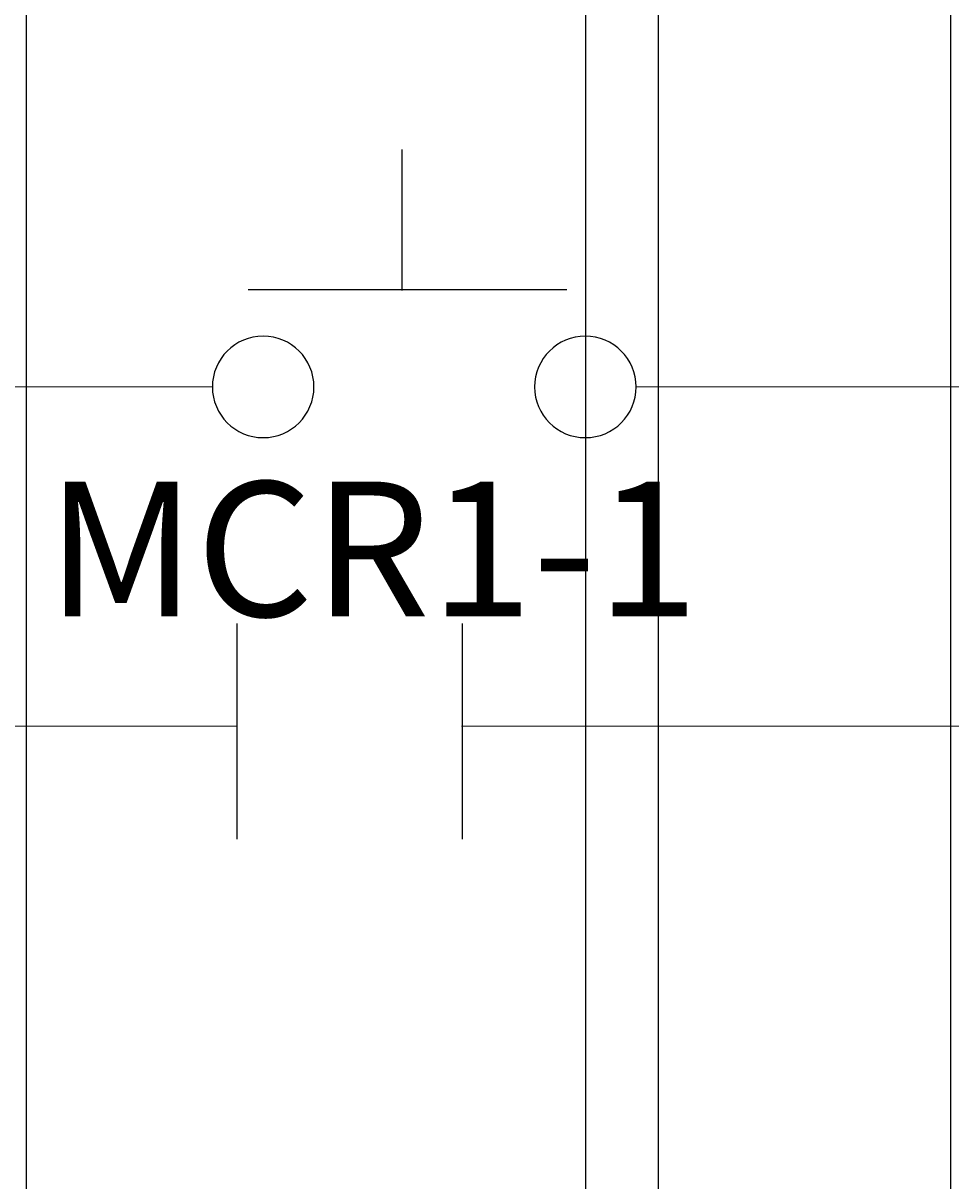
# Model space of a CAD drawing. Units: inches. Extents: x 738 to 1068, y 378 to 757.
# Tile 28 of 41: x 856 to 901, y 492 to 549. Entities that reach past the tile are written whole.
import ezdxf

# ---------------------------------------------------------------- set-up
doc = ezdxf.new("R2010")
doc.units = ezdxf.units.IN
doc.header["$MEASUREMENT"] = 0
for name, color, linetype, lineweight in [('A-ANNO-DIMS', 2, 'Continuous', 18), ('E-ANNO-TEXT', 7, 'Continuous', 18), ('E-CTRL-CONT', 4, 'Continuous', 25), ('E-CTRL-PBTN', 4, 'Continuous', 25), ('E-CTRL-WIRE', 7, 'Continuous', 18)]:
    doc.layers.add(name, color=color, linetype=linetype, lineweight=lineweight)
doc.styles.get("Standard").update_dxf_attribs({"font": 'arial.ttf'})
doc.dimstyles.get("Standard").update_dxf_attribs({"dimtxt": 0.18, "dimasz": 0.18, "dimexe": 0.18, "dimexo": 0.0625, "dimgap": 0.09, "dimtad": 0, "dimtih": 1, "dimtoh": 1, "dimdec": 4, "dimzin": 0, "dimdsep": 46, "dimtxsty": 'Standard', "dimcen": 0.09, "dimadec": 0, "dimazin": 0, "dimtfac": 1, "dimtdec": 4, "dimtofl": 0, "dimtmove": 0, "dimatfit": 3, "dimfxl": 1, "dimtolj": 1, "dimtzin": 0, "dimarcsym": 0})

# ---------------------------------------------------------------- blocks, each defined once
blk = doc.blocks.new('PB-ENABLE-NO')
for p, q in [((9.342, 7.241), (9.342, 14.19)), ((1.764, 7.299), (17.45, 7.299))]:
    blk.add_line(p, q)
for points in [[(0, 2.5, 1), (5, 2.5, 1)], [(15.861, 2.5, 1), (20.861, 2.5, 1)]]:
    blk.add_lwpolyline(points, format="xyb", close=True)
blk = doc.blocks.new('MCR-HOLD-CONTACT-NO')
for p, q in [((0, 0), (0, 10.627)), ((11.061, 10.627), (11.061, 0))]:
    blk.add_line(p, q)
blk = doc.blocks.new('*D27')
at = {"layer": 'A-ANNO-DIMS', "color": 0, "lineweight": -2, "transparency": 16777216}
for p, q in [((883.457, 646.923), (883.457, 378.239)), ((923.511, 646.923), (923.511, 378.239)), ((883.637, 378.419), (903.086, 378.419)), ((923.331, 378.419), (903.882, 378.419))]:
    blk.add_line(p, q, dxfattribs=at)
at = {"layer": 'A-ANNO-DIMS', "color": 0, "transparency": 16777216}
for points in [[(883.637, 378.449), (883.637, 378.389), (883.457, 378.419)], [(923.331, 378.449), (923.331, 378.389), (923.511, 378.419)]]:
    blk.add_solid(points, dxfattribs=at)
at = {"layer": 'Defpoints', "color": 0, "transparency": 16777216}
for p in [(883.457, 646.985), (923.511, 646.985), (923.511, 378.419)]:
    blk.add_point(p, dxfattribs=at)
at = {"layer": 'A-ANNO-DIMS', "color": 0, "transparency": 16777216, "insert": (903.484, 378.419), "char_height": 0.18, "attachment_point": 5}
blk.add_mtext('\\A1;40.05', dxfattribs=at)
blk = doc.blocks.new('*D33')
at = {"layer": 'A-ANNO-DIMS', "color": 0, "lineweight": -2, "transparency": 16777216}
for p, q in [((836.324, 514.624), (836.324, 378.239)), ((907.171, 514.624), (907.171, 378.239)), ((836.504, 378.419), (871.354, 378.419)), ((906.991, 378.419), (872.141, 378.419))]:
    blk.add_line(p, q, dxfattribs=at)
at = {"layer": 'A-ANNO-DIMS', "color": 0, "transparency": 16777216}
for points in [[(836.504, 378.449), (836.504, 378.389), (836.324, 378.419)], [(906.991, 378.449), (906.991, 378.389), (907.171, 378.419)]]:
    blk.add_solid(points, dxfattribs=at)
at = {"layer": 'Defpoints', "color": 0, "transparency": 16777216}
for p in [(836.324, 514.687), (907.171, 514.687), (907.171, 378.419)]:
    blk.add_point(p, dxfattribs=at)
at = {"layer": 'A-ANNO-DIMS', "color": 0, "transparency": 16777216, "insert": (871.748, 378.419), "char_height": 0.18, "attachment_point": 5}
blk.add_mtext('\\A1;70.85', dxfattribs=at)
blk = doc.blocks.new('*D35')
at = {"layer": 'A-ANNO-DIMS', "color": 0, "lineweight": -2, "transparency": 16777216}
for p, q in [((855.932, 686.266), (855.932, 378.239)), ((901.429, 686.267), (901.429, 378.239)), ((856.112, 378.419), (878.352, 378.419)), ((901.249, 378.419), (879.009, 378.419))]:
    blk.add_line(p, q, dxfattribs=at)
at = {"layer": 'A-ANNO-DIMS', "color": 0, "transparency": 16777216}
for points in [[(856.112, 378.449), (856.112, 378.389), (855.932, 378.419)], [(901.249, 378.449), (901.249, 378.389), (901.429, 378.419)]]:
    blk.add_solid(points, dxfattribs=at)
at = {"layer": 'Defpoints', "color": 0, "transparency": 16777216}
for p in [(855.932, 686.329), (901.429, 686.329), (901.429, 378.419)]:
    blk.add_point(p, dxfattribs=at)
at = {"layer": 'A-ANNO-DIMS', "color": 0, "transparency": 16777216, "insert": (878.68, 378.419), "char_height": 0.18, "attachment_point": 5}
blk.add_mtext('\\A1;45.5', dxfattribs=at)
blk = doc.blocks.new('*D38')
at = {"layer": 'A-ANNO-DIMS', "color": 0, "lineweight": -2, "transparency": 16777216}
for p, q in [((781.485, 593.017), (781.485, 378.239)), ((887.04, 593.067), (887.04, 378.239)), ((781.665, 378.419), (833.807, 378.419)), ((886.86, 378.419), (834.718, 378.419))]:
    blk.add_line(p, q, dxfattribs=at)
at = {"layer": 'A-ANNO-DIMS', "color": 0, "transparency": 16777216}
for points in [[(781.665, 378.449), (781.665, 378.389), (781.485, 378.419)], [(886.86, 378.449), (886.86, 378.389), (887.04, 378.419)]]:
    blk.add_solid(points, dxfattribs=at)
at = {"layer": 'Defpoints', "color": 0, "transparency": 16777216}
for p in [(781.485, 593.08), (887.04, 593.13), (887.04, 378.419)]:
    blk.add_point(p, dxfattribs=at)
at = {"layer": 'A-ANNO-DIMS', "color": 0, "transparency": 16777216, "insert": (834.263, 378.419), "char_height": 0.18, "attachment_point": 5}
blk.add_mtext('\\A1;105.56', dxfattribs=at)
blk = doc.blocks.new('*D39')
at = {"layer": 'A-ANNO-DIMS', "color": 0, "lineweight": -2, "transparency": 16777216}
for p, q in [((887.04, 581.418), (887.04, 378.239)), ((938.455, 581.418), (938.455, 378.239)), ((887.22, 378.419), (912.371, 378.419)), ((938.275, 378.419), (913.124, 378.419))]:
    blk.add_line(p, q, dxfattribs=at)
at = {"layer": 'A-ANNO-DIMS', "color": 0, "transparency": 16777216}
for points in [[(887.22, 378.449), (887.22, 378.389), (887.04, 378.419)], [(938.275, 378.449), (938.275, 378.389), (938.455, 378.419)]]:
    blk.add_solid(points, dxfattribs=at)
at = {"layer": 'Defpoints', "color": 0, "transparency": 16777216}
for p in [(887.04, 581.481), (938.455, 581.481), (938.455, 378.419)]:
    blk.add_point(p, dxfattribs=at)
at = {"layer": 'A-ANNO-DIMS', "color": 0, "transparency": 16777216, "insert": (912.748, 378.419), "char_height": 0.18, "attachment_point": 5}
blk.add_mtext('\\A1;51.41', dxfattribs=at)

msp = doc.modelspace()

# ---------------------------------------------------------------- linework, layer by layer
at = {"layer": 'E-CTRL-WIRE'}
for p, q in [((809.3803, 531.4009), (865.0964, 531.4009)), ((885.9574, 531.4009), (966.9395, 531.4009)), ((866.3244, 514.6866), (836.3244, 514.6866)), ((877.3586, 514.6866), (907.3586, 514.6866))]:
    msp.add_line(p, q, dxfattribs=at)

# ---------------------------------------------------------------- block references
at = {"layer": 'E-CTRL-CONT'}
msp.add_blockref('MCR-HOLD-CONTACT-NO', (866.324, 509.125), dxfattribs=at)
at = {"layer": 'E-CTRL-PBTN'}
msp.add_blockref('PB-ENABLE-NO', (865.096, 528.901), dxfattribs=at)

# ---------------------------------------------------------------- texts
at = {"layer": 'E-ANNO-TEXT'}
msp.add_text('MCR1-1', height=6.64426, dxfattribs=at).set_placement((856.923, 520.0926))

# ---------------------------------------------------------------- dimensions: what is measured, and where the dimension line sits
at = {"layer": 'A-ANNO-DIMS'}
for base, p1, p2, override, picture, middle in [((901.4286, 378.4191), (855.9323, 686.329), (901.4286, 686.3292), {"dimdec": 1, "dimlfac": 1, "dimrnd": 0, "dimzin": 0, "dimdsep": 46, "dimlunit": 2}, '*D35', (878.6804, 378.4191)), ((923.5105, 378.4191), (883.4574, 646.9853), (923.5105, 646.9853), {"dimdec": 2, "dimlfac": 1, "dimrnd": 0, "dimzin": 0, "dimdsep": 46, "dimlunit": 2}, '*D27', (903.484, 378.4191)), ((887.0404, 378.4191), (781.4846, 593.0796), (887.0404, 593.1296), {"dimdec": 2, "dimlfac": 1, "dimrnd": 0, "dimzin": 0, "dimdsep": 46, "dimlunit": 2}, '*D38', (834.2625, 378.4191)), ((938.455, 378.4191), (887.0404, 581.4808), (938.455, 581.4808), {"dimdec": 2, "dimlfac": 1, "dimrnd": 0, "dimzin": 0, "dimdsep": 46, "dimlunit": 2}, '*D39', (912.7477, 378.4191)), ((907.1708, 378.4191), (836.3244, 514.6866), (907.1708, 514.6866), {"dimdec": 2, "dimlfac": 1, "dimrnd": 0, "dimzin": 0, "dimdsep": 46, "dimlunit": 2}, '*D33', (871.7476, 378.4191))]:
    dim = msp.add_linear_dim(base=base, p1=p1, p2=p2, dimstyle='Standard', override=override, dxfattribs=at)
    dim.commit()
    dim.dimension.update_dxf_attribs({"geometry": picture, "text_midpoint": middle})

doc.saveas('drawing.dxf')
